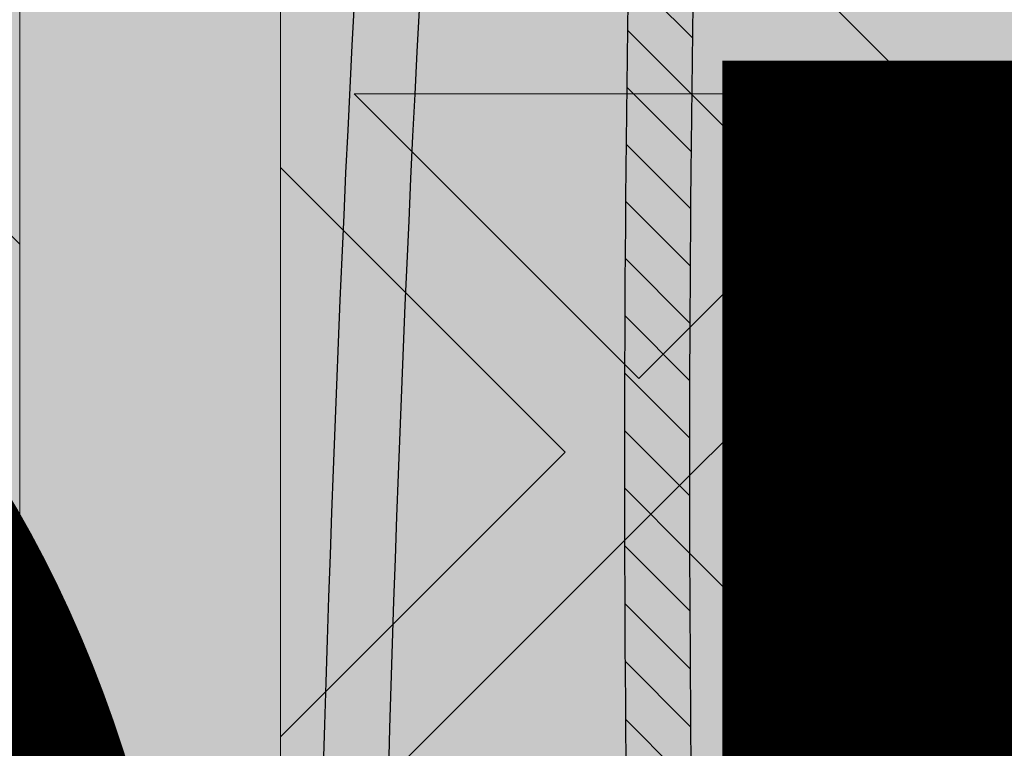
# Model space of a CAD drawing. Units: inches. Extents: x 844 to 2234, y 346 to 1084.
# Tile 77 of 93: x 1998.757 to 2001.166, y 702.727 to 704.51. Entities that reach past the tile are written whole.
import ezdxf

# ---------------------------------------------------------------- set-up
doc = ezdxf.new("R2010")
doc.units = ezdxf.units.IN
doc.header["$MEASUREMENT"] = 0
for name, color, linetype, lineweight in [('A-ANNO-DIMS', 2, 'Continuous', 18), ('furniture', 8, 'Continuous', 18), ('RA-AP-01$0$INT', 35, 'Continuous', 5)]:
    doc.layers.add(name, color=color, linetype=linetype, lineweight=lineweight)
doc.layers.add('RA-AP-01$0$FURN', color=3, linetype='Continuous')
doc.layers.add('RA-AP-01$0$WOOD', color=64, linetype='Continuous')
doc.styles.get("Standard").update_dxf_attribs({"font": 'arial.ttf'})
doc.dimstyles.get("Standard").update_dxf_attribs({"dimtxt": 6, "dimasz": 3, "dimexe": 0.18, "dimexo": 0.0625, "dimgap": 0.09, "dimtad": 0, "dimtih": 1, "dimtoh": 1, "dimdec": 1, "dimzin": 0, "dimdsep": 46, "dimlunit": 3, "dimtxsty": 'Standard', "dimblk": 'ARCHTICK', "dimcen": 0.09, "dimadec": 0, "dimazin": 0, "dimtfac": 1, "dimtdec": 1, "dimtofl": 0, "dimtmove": 0, "dimatfit": 3, "dimfxl": 1, "dimtolj": 1, "dimtzin": 0, "dimarcsym": 0})

# ---------------------------------------------------------------- blocks, each defined once
blk = doc.blocks.new('A$C18D01794')
at = {"layer": 'RA-AP-01$0$INT'}
h = blk.add_hatch(color=256, dxfattribs=at)
h.paths.add_polyline_path([(4.50521, -7.5855), (4.46935, -7.54964), (4.50521, -7.51378), (4.50521, -7.38196), (4.46935, -7.34611), (4.50521, -7.31025), (4.50521, -7.17843), (4.46935, -7.14257), (4.50521, -7.10671), (4.47692, -7.10671), (4.45521, -7.12843), (4.43349, -7.10671), (4.40521, -7.10671), (4.44106, -7.14257), (4.40521, -7.17843), (4.40521, -7.31025), (4.44106, -7.34611), (4.40521, -7.38196), (4.40521, -7.51378), (4.44106, -7.54964), (4.40521, -7.5855), (4.40521, -7.71732), (4.44106, -7.75318), (4.40521, -7.78903), (4.40521, -8.00671), (4.64435, -8.00671), (4.68021, -7.97085), (4.71606, -8.00671), (4.86935, -8.00671), (4.90521, -7.97085), (4.94106, -8.00671), (5.09435, -8.00671), (5.13021, -7.97085), (5.16606, -8.00671), (5.40521, -8.00671), (5.40521, -7.78903), (5.36935, -7.75318), (5.40521, -7.71732), (5.40521, -7.5855), (5.36935, -7.54964), (5.40521, -7.51378), (5.40521, -7.38196), (5.36935, -7.34611), (5.40521, -7.31025), (5.40521, -7.17843), (5.36935, -7.14257), (5.40521, -7.10671), (5.37692, -7.10671), (5.35521, -7.12843), (5.33349, -7.10671), (5.30521, -7.10671), (5.34106, -7.14257), (5.30521, -7.17843), (5.30521, -7.31025), (5.34106, -7.34611), (5.30521, -7.38196), (5.30521, -7.51378), (5.34106, -7.54964), (5.30521, -7.5855), (5.30521, -7.71732), (5.34106, -7.75318), (5.30521, -7.78903), (5.30521, -7.90671), (5.16606, -7.90671), (5.13021, -7.94257), (5.09435, -7.90671), (4.94106, -7.90671), (4.90521, -7.94257), (4.86935, -7.90671), (4.71606, -7.90671), (4.68021, -7.94257), (4.64435, -7.90671), (4.50521, -7.90671), (4.50521, -7.78903), (4.46935, -7.75318), (4.50521, -7.71732)])
h.paths.add_polyline_path([(4.48521, -7.70903), (4.45521, -7.73903), (4.42521, -7.70903), (4.42521, -7.59378), (4.45521, -7.56378), (4.48521, -7.59378)], flags=16)
h.paths.add_polyline_path([(4.45521, -7.76732), (4.48521, -7.79732), (4.48521, -7.91257), (4.45521, -7.94257), (4.42521, -7.91257), (4.42521, -7.79732)], flags=16)
h.paths.add_polyline_path([(4.45521, -7.5355), (4.42521, -7.5055), (4.42521, -7.39025), (4.45521, -7.36025), (4.48521, -7.39025), (4.48521, -7.5055)], flags=16)
h.paths.add_polyline_path([(4.49935, -7.92671), (4.63606, -7.92671), (4.66606, -7.95671), (4.63606, -7.98671), (4.49935, -7.98671), (4.46935, -7.95671)], flags=16)
h.paths.add_polyline_path([(4.42521, -7.94085), (4.47106, -7.98671), (4.42521, -7.98671)], flags=16)
h.paths.add_polyline_path([(4.45521, -7.33196), (4.42521, -7.30196), (4.42521, -7.18671), (4.45521, -7.15671), (4.48521, -7.18671), (4.48521, -7.30196)], flags=16)
h.paths.add_polyline_path([(4.72435, -7.92671), (4.86106, -7.92671), (4.89106, -7.95671), (4.86106, -7.98671), (4.72435, -7.98671), (4.69435, -7.95671)], flags=16)
h.paths.add_polyline_path([(4.91935, -7.95671), (4.94935, -7.92671), (5.08606, -7.92671), (5.11606, -7.95671), (5.08606, -7.98671), (4.94935, -7.98671)], flags=16)
h.paths.add_polyline_path([(5.14435, -7.95671), (5.17435, -7.92671), (5.31106, -7.92671), (5.34106, -7.95671), (5.31106, -7.98671), (5.17435, -7.98671)], flags=16)
h.paths.add_polyline_path([(5.32521, -7.59378), (5.35521, -7.56378), (5.38521, -7.59378), (5.38521, -7.70903), (5.35521, -7.73903), (5.32521, -7.70903)], flags=16)
h.paths.add_polyline_path([(5.32521, -7.79732), (5.35521, -7.76732), (5.38521, -7.79732), (5.38521, -7.91257), (5.35521, -7.94257), (5.32521, -7.91257)], flags=16)
h.paths.add_polyline_path([(5.32521, -7.5055), (5.32521, -7.39025), (5.35521, -7.36025), (5.38521, -7.39025), (5.38521, -7.5055), (5.35521, -7.5355)], flags=16)
h.paths.add_polyline_path([(5.32521, -7.30196), (5.32521, -7.18671), (5.35521, -7.15671), (5.38521, -7.18671), (5.38521, -7.30196), (5.35521, -7.33196)], flags=16)
h.paths.add_polyline_path([(5.33935, -7.98671), (5.38521, -7.94085), (5.38521, -7.98671)], flags=16)
h = blk.add_hatch(color=256, dxfattribs=at)
h.paths.add_polyline_path([(4.46935, -7.14257), (4.50521, -7.17843), (4.50521, -7.10671)])
h.paths.add_polyline_path([(4.45521, -7.12843), (4.47692, -7.10671), (4.43349, -7.10671)])
h.paths.add_polyline_path([(4.40521, -7.17843), (4.44106, -7.14257), (4.40521, -7.10671)])
h.paths.add_polyline_path([(4.42521, -7.30196), (4.45521, -7.33196), (4.48521, -7.30196), (4.48521, -7.18671), (4.45521, -7.15671), (4.42521, -7.18671)])
h.paths.add_polyline_path([(4.50521, -7.38196), (4.50521, -7.31025), (4.46935, -7.34611)])
h.paths.add_polyline_path([(4.42521, -7.5055), (4.45521, -7.5355), (4.48521, -7.5055), (4.48521, -7.39025), (4.45521, -7.36025), (4.42521, -7.39025)])
h.paths.add_polyline_path([(4.42521, -7.70903), (4.45521, -7.73903), (4.48521, -7.70903), (4.48521, -7.59378), (4.45521, -7.56378), (4.42521, -7.59378)])
h.paths.add_polyline_path([(4.46935, -7.54964), (4.50521, -7.5855), (4.50521, -7.51378)])
h.paths.add_polyline_path([(4.40521, -7.5855), (4.44106, -7.54964), (4.40521, -7.51378)])
h.paths.add_polyline_path([(4.40521, -7.78903), (4.44106, -7.75318), (4.40521, -7.71732)])
h.paths.add_polyline_path([(4.46935, -7.75318), (4.50521, -7.78903), (4.50521, -7.71732)])
h.paths.add_polyline_path([(4.42521, -7.91257), (4.45521, -7.94257), (4.48521, -7.91257), (4.48521, -7.79732), (4.45521, -7.76732), (4.42521, -7.79732)])
h.paths.add_polyline_path([(4.42521, -7.98671), (4.47106, -7.98671), (4.42521, -7.94085)])
h.paths.add_polyline_path([(4.49935, -7.98671), (4.63606, -7.98671), (4.66606, -7.95671), (4.63606, -7.92671), (4.49935, -7.92671), (4.46935, -7.95671)])
h.paths.add_polyline_path([(4.68021, -7.94257), (4.71606, -7.90671), (4.64435, -7.90671)])
h.paths.add_polyline_path([(4.64435, -8.00671), (4.71606, -8.00671), (4.68021, -7.97085)])
h.paths.add_polyline_path([(4.72435, -7.98671), (4.86106, -7.98671), (4.89106, -7.95671), (4.86106, -7.92671), (4.72435, -7.92671), (4.69435, -7.95671)])
h.paths.add_polyline_path([(4.90521, -7.94257), (4.94106, -7.90671), (4.86935, -7.90671)])
h.paths.add_polyline_path([(4.86935, -8.00671), (4.94106, -8.00671), (4.90521, -7.97085)])
h.paths.add_polyline_path([(4.94935, -7.98671), (5.08606, -7.98671), (5.11606, -7.95671), (5.08606, -7.92671), (4.94935, -7.92671), (4.91935, -7.95671)])
h.paths.add_polyline_path([(5.13021, -7.94257), (5.16606, -7.90671), (5.09435, -7.90671)])
h.paths.add_polyline_path([(5.09435, -8.00671), (5.16606, -8.00671), (5.13021, -7.97085)])
h.paths.add_polyline_path([(5.17435, -7.98671), (5.31106, -7.98671), (5.34106, -7.95671), (5.31106, -7.92671), (5.17435, -7.92671), (5.14435, -7.95671)])
h.paths.add_polyline_path([(5.32521, -7.91257), (5.35521, -7.94257), (5.38521, -7.91257), (5.38521, -7.79732), (5.35521, -7.76732), (5.32521, -7.79732)])
h.paths.add_polyline_path([(5.33935, -7.98671), (5.38521, -7.98671), (5.38521, -7.94085)])
h.paths.add_polyline_path([(5.32521, -7.70903), (5.35521, -7.73903), (5.38521, -7.70903), (5.38521, -7.59378), (5.35521, -7.56378), (5.32521, -7.59378)])
h.paths.add_polyline_path([(5.30521, -7.78903), (5.34106, -7.75318), (5.30521, -7.71732)])
h.paths.add_polyline_path([(5.36935, -7.75318), (5.40521, -7.78903), (5.40521, -7.71732)])
h.paths.add_polyline_path([(5.40521, -7.5855), (5.40521, -7.51378), (5.36935, -7.54964)])
h.paths.add_polyline_path([(5.30521, -7.5855), (5.34106, -7.54964), (5.30521, -7.51378)])
h.paths.add_polyline_path([(5.32521, -7.5055), (5.35521, -7.5355), (5.38521, -7.5055), (5.38521, -7.39025), (5.35521, -7.36025), (5.32521, -7.39025)])
h.paths.add_polyline_path([(5.30521, -7.38196), (5.34106, -7.34611), (5.30521, -7.31025)])
h.paths.add_polyline_path([(5.32521, -7.30196), (5.35521, -7.33196), (5.38521, -7.30196), (5.38521, -7.18671), (5.35521, -7.15671), (5.32521, -7.18671)])
h.paths.add_polyline_path([(5.40458, -7.38134, -0.001218), (5.40521, -7.38111), (5.40521, -7.31025), (5.36935, -7.34611)])
h.paths.add_polyline_path([(5.36935, -7.14257), (5.40521, -7.17843), (5.40521, -7.10671)])
h.paths.add_polyline_path([(5.35521, -7.12843), (5.37692, -7.10671), (5.33349, -7.10671)])
h.paths.add_polyline_path([(5.30521, -7.17843), (5.34106, -7.14257), (5.30521, -7.10671)])
blk.add_hatch(color=256, dxfattribs=at).paths.add_polyline_path([(4.50521, -7.90671), (5.30521, -7.90671), (5.30521, -7.10671), (5.25521, -7.10671), (5.25521, -7.85671), (4.55521, -7.85671), (4.55521, -7.10671), (4.50521, -7.10671)])
h = blk.add_hatch(color=256, dxfattribs=at)
h.paths.add_polyline_path([(4.58592, -7.85671), (4.6142, -7.85671), (4.66885, -7.80207), (4.72349, -7.85671), (4.77177, -7.85671), (4.82642, -7.80207), (4.86278, -7.83843), (4.8445, -7.85671), (4.86278, -7.85671), (4.90521, -7.81429), (4.94763, -7.85671), (4.96592, -7.85671), (4.94763, -7.83843), (4.98399, -7.80207), (5.03864, -7.85671), (5.08692, -7.85671), (5.14157, -7.80207), (5.19621, -7.85671), (5.2245, -7.85671), (4.90521, -7.53742)])
h.paths.add_polyline_path([(4.89521, -7.57571), (4.89521, -7.685), (4.84056, -7.63035)], flags=16)
h.paths.add_polyline_path([(4.91521, -7.57571), (4.96985, -7.63035), (4.91521, -7.685)], flags=16)
h.paths.add_polyline_path([(4.82642, -7.64449), (4.88106, -7.69914), (4.77177, -7.69914)], flags=16)
h.paths.add_polyline_path([(4.98399, -7.64449), (5.03864, -7.69914), (4.92935, -7.69914)], flags=16)
h.paths.add_polyline_path([(4.88106, -7.71914), (4.82642, -7.77378), (4.77177, -7.71914)], flags=16)
h.paths.add_polyline_path([(4.92935, -7.71914), (5.03864, -7.71914), (4.98399, -7.77378)], flags=16)
h.paths.add_polyline_path([(4.89521, -7.73328), (4.89521, -7.806), (4.87692, -7.82429), (4.84056, -7.78793)], flags=16)
h.paths.add_polyline_path([(4.91521, -7.73328), (4.96985, -7.78793), (4.93349, -7.82429), (4.91521, -7.806)], flags=16)
h.paths.add_polyline_path([(4.75763, -7.73328), (4.81228, -7.78793), (4.75763, -7.84257)], flags=16)
h.paths.add_polyline_path([(4.73763, -7.73328), (4.73763, -7.84257), (4.68299, -7.78793)], flags=16)
h.paths.add_polyline_path([(5.05278, -7.73328), (5.05278, -7.84257), (4.99814, -7.78793)], flags=16)
h.paths.add_polyline_path([(5.07278, -7.73328), (5.12742, -7.78793), (5.07278, -7.84257)], flags=16)
h.paths.add_polyline_path([(4.93592, -7.50671), (5.25521, -7.826), (5.25521, -7.79772), (5.20056, -7.74307), (5.25521, -7.68843), (5.25521, -7.64014), (5.20056, -7.5855), (5.23692, -7.54914), (5.25521, -7.56742), (5.25521, -7.54914), (5.21278, -7.50671), (5.25521, -7.46429), (5.25521, -7.446), (5.23692, -7.46429), (5.20056, -7.42793), (5.25521, -7.37328), (5.25521, -7.325), (5.20056, -7.27035), (5.25521, -7.21571), (5.25521, -7.18742)])
h.paths.add_polyline_path([(5.04299, -7.42793), (5.09763, -7.37328), (5.09763, -7.48257)], flags=16)
h.paths.add_polyline_path([(5.02885, -7.44207), (5.08349, -7.49671), (4.9742, -7.49671)], flags=16)
h.paths.add_polyline_path([(5.11763, -7.37328), (5.17228, -7.42793), (5.11763, -7.48257)], flags=16)
h.paths.add_polyline_path([(5.08349, -7.51671), (5.02885, -7.57136), (4.9742, -7.51671)], flags=16)
h.paths.add_polyline_path([(5.13177, -7.35914), (5.18642, -7.41378), (5.24106, -7.35914)], flags=17)
h.paths.add_polyline_path([(5.13177, -7.49671), (5.18642, -7.44207), (5.22278, -7.47843), (5.2045, -7.49671)], flags=16)
h.paths.add_polyline_path([(5.09763, -7.53085), (5.09763, -7.64014), (5.04299, -7.5855)], flags=16)
h.paths.add_polyline_path([(5.13177, -7.33914), (5.24106, -7.33914), (5.18642, -7.28449)], flags=17)
h.paths.add_polyline_path([(5.13177, -7.51671), (5.2045, -7.51671), (5.22278, -7.535), (5.18642, -7.57136)], flags=16)
h.paths.add_polyline_path([(5.11763, -7.53085), (5.17228, -7.5855), (5.11763, -7.64014)], flags=16)
h.paths.add_polyline_path([(5.18642, -7.59964), (5.24106, -7.65429), (5.13177, -7.65429)], flags=16)
h.paths.add_polyline_path([(5.13177, -7.67429), (5.24106, -7.67429), (5.18642, -7.72893)], flags=16)
h.paths.add_polyline_path([(5.25521, -7.126), (5.25521, -7.10671), (4.55521, -7.10671), (4.55521, -7.126), (4.90521, -7.476)])
h.paths.add_polyline_path([(4.98399, -7.36893), (4.92935, -7.31429), (5.03864, -7.31429)], flags=16)
h.paths.add_polyline_path([(4.96985, -7.38307), (4.91521, -7.43772), (4.91521, -7.32843)], flags=16)
h.paths.add_polyline_path([(4.92935, -7.29429), (4.98399, -7.23964), (5.03864, -7.29429)], flags=16)
h.paths.add_polyline_path([(5.05278, -7.28014), (4.99814, -7.2255), (5.05278, -7.17085)], flags=16)
h.paths.add_polyline_path([(5.07278, -7.28014), (5.07278, -7.17085), (5.12742, -7.2255)], flags=16)
h.paths.add_polyline_path([(4.89521, -7.43772), (4.84056, -7.38307), (4.89521, -7.32843)], flags=16)
h.paths.add_polyline_path([(4.91521, -7.28014), (4.91521, -7.20742), (4.93349, -7.18914), (4.96985, -7.2255)], flags=16)
h.paths.add_polyline_path([(4.88106, -7.31429), (4.82642, -7.36893), (4.77177, -7.31429)], flags=16)
h.paths.add_polyline_path([(4.89521, -7.28014), (4.84056, -7.2255), (4.87692, -7.18914), (4.89521, -7.20742)], flags=16)
h.paths.add_polyline_path([(4.98399, -7.21136), (4.94763, -7.175), (4.96592, -7.15671), (5.03864, -7.15671)], flags=16)
h.paths.add_polyline_path([(4.88106, -7.29429), (4.77177, -7.29429), (4.82642, -7.23964)], flags=16)
h.paths.add_polyline_path([(4.90521, -7.19914), (4.86278, -7.15671), (4.94763, -7.15671)], flags=16)
h.paths.add_polyline_path([(5.14157, -7.21136), (5.08692, -7.15671), (5.19621, -7.15671)], flags=16)
h.paths.add_polyline_path([(4.82642, -7.21136), (4.77177, -7.15671), (4.8445, -7.15671), (4.86278, -7.175)], flags=16)
h.paths.add_polyline_path([(4.81228, -7.2255), (4.75763, -7.28014), (4.75763, -7.17085)], flags=16)
h.paths.add_polyline_path([(4.73763, -7.28014), (4.68299, -7.2255), (4.73763, -7.17085)], flags=16)
h.paths.add_polyline_path([(4.72349, -7.15671), (4.66885, -7.21136), (4.6142, -7.15671)], flags=16)
h.paths.add_polyline_path([(4.59763, -7.50671), (4.55521, -7.54914), (4.55521, -7.56742), (4.57349, -7.54914), (4.60985, -7.5855), (4.55521, -7.64014), (4.55521, -7.68843), (4.60985, -7.74307), (4.55521, -7.79772), (4.55521, -7.826), (4.8745, -7.50671), (4.55521, -7.18742), (4.55521, -7.21571), (4.60985, -7.27035), (4.55521, -7.325), (4.55521, -7.37328), (4.60985, -7.42793), (4.57349, -7.46429), (4.55521, -7.446), (4.55521, -7.46429)])
h.paths.add_polyline_path([(4.71278, -7.48257), (4.71278, -7.37328), (4.76742, -7.42793)], flags=16)
h.paths.add_polyline_path([(4.72692, -7.49671), (4.78157, -7.44207), (4.83621, -7.49671)], flags=16)
h.paths.add_polyline_path([(4.69278, -7.48257), (4.63814, -7.42793), (4.69278, -7.37328)], flags=16)
h.paths.add_polyline_path([(4.72692, -7.51671), (4.83621, -7.51671), (4.78157, -7.57136)], flags=16)
h.paths.add_polyline_path([(4.67864, -7.49671), (4.60592, -7.49671), (4.58763, -7.47843), (4.62399, -7.44207)], flags=16)
h.paths.add_polyline_path([(4.71278, -7.53085), (4.76742, -7.5855), (4.71278, -7.64014)], flags=16)
h.paths.add_polyline_path([(4.67864, -7.51671), (4.62399, -7.57136), (4.58763, -7.535), (4.60592, -7.51671)], flags=16)
h.paths.add_polyline_path([(4.69278, -7.53085), (4.69278, -7.64014), (4.63814, -7.5855)], flags=16)
h.paths.add_polyline_path([(4.62399, -7.41378), (4.67864, -7.35914), (4.56935, -7.35914)], flags=17)
h.paths.add_polyline_path([(4.62399, -7.59964), (4.67864, -7.65429), (4.56935, -7.65429)], flags=16)
h.paths.add_polyline_path([(4.67864, -7.33914), (4.62399, -7.28449), (4.56935, -7.33914)], flags=17)
h.paths.add_polyline_path([(4.67864, -7.67429), (4.62399, -7.72893), (4.56935, -7.67429)], flags=16)
h = blk.add_hatch(color=256, dxfattribs=at)
h.paths.add_polyline_path([(4.90521, -7.53742), (4.8745, -7.50671), (4.55521, -7.826), (4.55521, -7.85671), (4.58592, -7.85671)])
h.paths.add_polyline_path([(4.93592, -7.50671), (4.90521, -7.53742), (5.2245, -7.85671), (5.25521, -7.85671), (5.25521, -7.826)])
h.paths.add_polyline_path([(5.25521, -7.18742), (5.25521, -7.126), (4.90521, -7.476), (4.93592, -7.50671)])
h.paths.add_polyline_path([(4.8745, -7.50671), (4.90521, -7.476), (4.55521, -7.126), (4.55521, -7.18742)])
h = blk.add_hatch(color=256, dxfattribs=at)
h.paths.add_polyline_path([(4.89521, -7.32843), (4.84056, -7.38307), (4.89521, -7.43772)])
h.paths.add_polyline_path([(4.91521, -7.43772), (4.96985, -7.38307), (4.91521, -7.32843)])
h.paths.add_polyline_path([(4.92935, -7.31429), (4.98399, -7.36893), (5.03864, -7.31429)])
h.paths.add_polyline_path([(5.03864, -7.29429), (4.98399, -7.23964), (4.92935, -7.29429)])
h.paths.add_polyline_path([(4.96985, -7.2255), (4.93349, -7.18914), (4.91521, -7.20742), (4.91521, -7.28014)])
h.paths.add_polyline_path([(4.96592, -7.15671), (4.94763, -7.175), (4.98399, -7.21136), (5.03864, -7.15671)])
h.paths.add_polyline_path([(4.99814, -7.2255), (5.05278, -7.28014), (5.05278, -7.17085)])
h.paths.add_polyline_path([(5.07278, -7.28014), (5.12742, -7.2255), (5.07278, -7.17085)])
h.paths.add_polyline_path([(5.19621, -7.15671), (5.08692, -7.15671), (5.14157, -7.21136)])
h.paths.add_polyline_path([(4.86278, -7.15671), (4.90521, -7.19914), (4.94763, -7.15671)])
h.paths.add_polyline_path([(4.89521, -7.28014), (4.89521, -7.20742), (4.87692, -7.18914), (4.84056, -7.2255)])
h.paths.add_polyline_path([(4.82642, -7.23964), (4.77177, -7.29429), (4.88106, -7.29429)])
h.paths.add_polyline_path([(4.77177, -7.31429), (4.82642, -7.36893), (4.88106, -7.31429)])
h.paths.add_polyline_path([(4.75763, -7.28014), (4.81228, -7.2255), (4.75763, -7.17085)])
h.paths.add_polyline_path([(4.86278, -7.175), (4.8445, -7.15671), (4.77177, -7.15671), (4.82642, -7.21136)])
h.paths.add_polyline_path([(4.68299, -7.2255), (4.73763, -7.28014), (4.73763, -7.17085)])
h.paths.add_polyline_path([(4.72349, -7.15671), (4.6142, -7.15671), (4.66885, -7.21136)])
h = blk.add_hatch(color=256, dxfattribs=at)
h.paths.add_polyline_path([(5.02885, -7.57136), (4.9742, -7.51671), (5.08349, -7.51671)])
h.paths.add_polyline_path([(4.9742, -7.49671), (5.02885, -7.44207), (5.08349, -7.49671)])
h.paths.add_polyline_path([(5.04299, -7.42793), (5.09763, -7.37328), (5.09763, -7.48257)])
h.paths.add_polyline_path([(5.11763, -7.48257), (5.11763, -7.37328), (5.17228, -7.42793)])
h.paths.add_polyline_path([(5.13177, -7.49671), (5.18642, -7.44207), (5.22278, -7.47843), (5.2045, -7.49671)])
h.paths.add_polyline_path([(5.23692, -7.46429), (5.20056, -7.42793), (5.25521, -7.37328), (5.25521, -7.446)])
h.paths.add_polyline_path([(5.18642, -7.41378), (5.13177, -7.35914), (5.24106, -7.35914)])
h.paths.add_polyline_path([(5.13177, -7.33914), (5.18642, -7.28449), (5.24106, -7.33914)])
h.paths.add_polyline_path([(5.20056, -7.27035), (5.25521, -7.21571), (5.25521, -7.325)])
h.paths.add_polyline_path([(5.21278, -7.50671), (5.25521, -7.46429), (5.25521, -7.54914)])
h.paths.add_polyline_path([(5.13177, -7.51671), (5.2045, -7.51671), (5.22278, -7.535), (5.18642, -7.57136)])
h.paths.add_polyline_path([(5.11763, -7.64014), (5.11763, -7.53085), (5.17228, -7.5855)])
h.paths.add_polyline_path([(5.04299, -7.5855), (5.09763, -7.53085), (5.09763, -7.64014)])
h.paths.add_polyline_path([(5.13177, -7.65429), (5.18642, -7.59964), (5.24106, -7.65429)])
h.paths.add_polyline_path([(5.20056, -7.5855), (5.23692, -7.54914), (5.25521, -7.56742), (5.25521, -7.64014)])
h.paths.add_polyline_path([(5.18642, -7.72893), (5.13177, -7.67429), (5.24106, -7.67429)])
h.paths.add_polyline_path([(5.20056, -7.74307), (5.25521, -7.68843), (5.25521, -7.79772)])
for p, q in [((5.25521, -7.10671), (5.25521, -7.85671)), ((4.90521, -7.476), (5.25521, -7.126)), ((5.07278, -7.17085), (5.12742, -7.2255)), ((4.93592, -7.50671), (5.25521, -7.18742)), ((5.25521, -7.21571), (5.20056, -7.27035)), ((5.25521, -7.325), (5.25521, -7.21571)), ((5.12742, -7.2255), (5.07278, -7.28014)), ((5.25521, -7.325), (5.20056, -7.27035)), ((5.18642, -7.28449), (5.13177, -7.33914)), ((5.24106, -7.33914), (5.18642, -7.28449)), ((5.30521, -7.31025), (5.34106, -7.34611)), ((5.13177, -7.33914), (5.24106, -7.33914))]:
    blk.add_line(p, q, dxfattribs=at)
blk.add_lwpolyline([(5.30521, -7.10671), (5.30521, -7.90671), (4.50521, -7.90671), (4.50521, -7.10671)], dxfattribs=at)
blk = doc.blocks.new('A$C32926AE1')
at = {"layer": 'RA-AP-01$0$WOOD'}
h = blk.add_hatch(color=256, dxfattribs=at)
h.dxf.hatch_style = 1
h.paths.add_polyline_path([(5.15743, 4.57348, -0.100949), (5.1554, 4.59337, -0.184266), (5.17225, 4.6388, 0.205661), (5.17956, 4.66132, 0.361434), (5.13435, 4.70652, 0.205661), (5.11183, 4.69921, -0.184266), (5.0664, 4.68237, -0.105531), (5.04566, 4.68467, 0.156764), (4.76389, 4.68467, -0.105531), (4.74314, 4.68237, -0.184266), (4.69771, 4.69921, 0.205661), (4.67519, 4.70652, 0.361434), (4.62998, 4.66132, 0.205661), (4.63729, 4.6388, -0.184266), (4.65414, 4.59337, -0.100949), (4.65211, 4.57348, 0.02141), (4.62975, 4.15671, 0.02141), (4.65211, 3.73994, -0.100949), (4.65414, 3.72006, -0.184266), (4.63729, 3.67463, 0.205661), (4.62998, 3.65211, 0.361434), (4.67519, 3.6069, 0.205661), (4.69771, 3.61421, -0.184266), (4.74314, 3.63106, -0.105531), (4.76389, 3.62875, 0.156764), (5.04566, 3.62875, -0.105531), (5.0664, 3.63106, -0.184266), (5.11183, 3.61421, 0.205661), (5.13435, 3.6069, 0.361434), (5.17956, 3.65211, 0.205661), (5.17225, 3.67463, -0.184266), (5.1554, 3.72006, -0.100949), (5.15743, 3.73994, 0.02141), (5.17979, 4.15671, 0.02141)])
h.paths.add_polyline_path([(4.63975, 4.15671, 0.021354), (4.66197, 3.74189, -0.094076), (4.66414, 3.71961, -0.182482), (4.64481, 3.66804, 0.205661), (4.63994, 3.65302, 0.361434), (4.67611, 3.61686, 0.205661), (4.69112, 3.62173, -0.182482), (4.7427, 3.64106, -0.102989), (4.76699, 3.63826, 0.156709), (5.04255, 3.63826, -0.102989), (5.06685, 3.64106, -0.182482), (5.11842, 3.62173, 0.205661), (5.13344, 3.61686, 0.361434), (5.1696, 3.65302, 0.205661), (5.16473, 3.66804, -0.182482), (5.1454, 3.71961, -0.094076), (5.14757, 3.74189, 0.021354), (5.16979, 4.15671, 0.021354), (5.14757, 4.57154, -0.094076), (5.1454, 4.59381, -0.182482), (5.16473, 4.64539, 0.205661), (5.1696, 4.6604, 0.361434), (5.13344, 4.69657, 0.205661), (5.11842, 4.69169, -0.182482), (5.06685, 4.67236, -0.102989), (5.04255, 4.67517, 0.156709), (4.76699, 4.67517, -0.102989), (4.7427, 4.67236, -0.182482), (4.69112, 4.69169, 0.205661), (4.67611, 4.69657, 0.361434), (4.63994, 4.6604, 0.205661), (4.64481, 4.64539, -0.182482), (4.66414, 4.59381, -0.094076), (4.66197, 4.57154, 0.021354)], flags=16)
h.paths.add_polyline_path([(5.12979, 4.43217, -0.014166), (5.13015, 4.15693, -0.014166), (5.12979, 3.88169, -0.078525), (5.1098, 3.75514, 0.094597), (5.10541, 3.7179, 0.104317), (5.11607, 3.67039, 0.104317), (5.06856, 3.68105, 0.094597), (5.03132, 3.67666, -0.158024), (4.77823, 3.67666, 0.094597), (4.74098, 3.68105, 0.104317), (4.69347, 3.67039, 0.104317), (4.70413, 3.7179, 0.094597), (4.69975, 3.75514, -0.078525), (4.67975, 3.88169, -0.014166), (4.67939, 4.15693, -0.014166), (4.67975, 4.43217, -0.078525), (4.69975, 4.55871, 0.094597), (4.70413, 4.59596, 0.104317), (4.69347, 4.64347, 0.104317), (4.74098, 4.6328, 0.094597), (4.77823, 4.63719, -0.158024), (5.03132, 4.63719, 0.094597), (5.06856, 4.6328, 0.104317), (5.11607, 4.64347, 0.104317), (5.10541, 4.59596, 0.094597), (5.1098, 4.55871, -0.078525)], flags=0)
h.paths.add_polyline_path([(5.11979, 4.43226, -0.0142), (5.12016, 4.15693, -0.0142), (5.11979, 3.8816, -0.078489), (5.10027, 3.75819, 0.094014), (5.09541, 3.71748, 0.060627), (5.09962, 3.68684, 0.060627), (5.06898, 3.69105, 0.094014), (5.02827, 3.68619, -0.158071), (4.78127, 3.68619, 0.094014), (4.74056, 3.69105, 0.060627), (4.70993, 3.68684, 0.060627), (4.71413, 3.71748, 0.094014), (4.70927, 3.75819, -0.078489), (4.68975, 3.8816, -0.0142), (4.68939, 4.15693, -0.0142), (4.68975, 4.43226, -0.078489), (4.70927, 4.55566, 0.094014), (4.71413, 4.59638, 0.060627), (4.70993, 4.62701, 0.060627), (4.74056, 4.62281, 0.094014), (4.78127, 4.62767, -0.158071), (5.02827, 4.62767, 0.094014), (5.06898, 4.62281, 0.060627), (5.09962, 4.62701, 0.060627), (5.09541, 4.59638, 0.094014), (5.10027, 4.55566, -0.078489)], flags=0)
h.paths.add_polyline_path([(5.06979, 4.43022, -0.014242), (5.07017, 4.15693, -0.014242), (5.06979, 3.88364, -0.080061), (5.05266, 3.77346, 0.052642), (5.04591, 3.74055, 0.052642), (5.013, 3.7338, -0.158303), (4.79655, 3.7338, 0.052642), (4.76363, 3.74055, 0.052642), (4.75688, 3.77346, -0.080061), (4.73975, 3.88364, -0.014242), (4.73937, 4.15693, -0.014242), (4.73975, 4.43022, -0.080061), (4.75688, 4.54039, 0.052642), (4.76363, 4.5733, 0.052642), (4.79655, 4.58006, -0.158303), (5.013, 4.58006, 0.052642), (5.04591, 4.5733, 0.052642), (5.05266, 4.54039, -0.080061)], flags=0)
h.paths.add_polyline_path([(5.04979, 4.43038, -0.01431), (5.05018, 4.15693, -0.01431), (5.04979, 3.88347, -0.080069), (5.03362, 3.77958, 0.030626), (5.02824, 3.75822, 0.030626), (5.00688, 3.75284, -0.158398), (4.80266, 3.75284, 0.030626), (4.7813, 3.75822, 0.030626), (4.77592, 3.77958, -0.080069), (4.75975, 3.88347, -0.01431), (4.75936, 4.15693, -0.01431), (4.75975, 4.43038, -0.080069), (4.77592, 4.53427, 0.030626), (4.7813, 4.55564, 0.030626), (4.80266, 4.56102, -0.158398), (5.00688, 4.56102, 0.030626), (5.02824, 4.55564, 0.030626), (5.03362, 4.53427, -0.080069)], flags=0)
h.paths.add_polyline_path([(4.99977, 4.42817, -0.014344), (5.0002, 4.15693, -0.014344), (4.99977, 3.88568, -0.078464), (4.98736, 3.7991, -0.150605), (4.82219, 3.7991, -0.078464), (4.80978, 3.88568, -0.014344), (4.80934, 4.15693, -0.014344), (4.80978, 4.42817, -0.078464), (4.82219, 4.51475, -0.150605), (4.98736, 4.51475, -0.078464)], flags=0)
h.paths.add_polyline_path([(4.97976, 4.42764, -0.014377), (4.98021, 4.15693, -0.014377), (4.97976, 3.88621, -0.068924), (4.97118, 3.81528, -0.129665), (4.83836, 3.81528, -0.068924), (4.82979, 3.88621, -0.014377), (4.82934, 4.15693, -0.014377), (4.82979, 4.42764, -0.068924), (4.83836, 4.49858, -0.129665), (4.97118, 4.49858, -0.068924)], flags=0)
h = blk.add_hatch(color=256, dxfattribs=at)
h.dxf.hatch_style = 1
h.paths.add_polyline_path([(5.1454, 4.59381, -0.182482), (5.16473, 4.64539, 0.205661), (5.1696, 4.6604, 0.361434), (5.13344, 4.69657, 0.205661), (5.11842, 4.69169, -0.182482), (5.06685, 4.67236, -0.102989), (5.04255, 4.67517, 0.156709), (4.76699, 4.67517, -0.102989), (4.7427, 4.67236, -0.182482), (4.69112, 4.69169, 0.205661), (4.67611, 4.69657, 0.361434), (4.63994, 4.6604, 0.205661), (4.64481, 4.64539, -0.182482), (4.66414, 4.59381, -0.094076), (4.66197, 4.57154, 0.021354), (4.63975, 4.15671, 0.021354), (4.66197, 3.74189, -0.094076), (4.66414, 3.71961, -0.182482), (4.64481, 3.66804, 0.205661), (4.63994, 3.65302, 0.361434), (4.67611, 3.61686, 0.205661), (4.69112, 3.62173, -0.182482), (4.7427, 3.64106, -0.102989), (4.76699, 3.63826, 0.156709), (5.04255, 3.63826, -0.102989), (5.06685, 3.64106, -0.182482), (5.11842, 3.62173, 0.205661), (5.13344, 3.61686, 0.361434), (5.1696, 3.65302, 0.205661), (5.16473, 3.66804, -0.182482), (5.1454, 3.71961, -0.094076), (5.14757, 3.74189, 0.021354), (5.16979, 4.15671, 0.021354), (5.14757, 4.57154, -0.094076)])
h.paths.add_polyline_path([(5.1098, 4.55871, -0.078525), (5.12979, 4.43217, -0.014166), (5.13015, 4.15693, -0.014166), (5.12979, 3.88169, -0.078525), (5.1098, 3.75514, 0.094597), (5.10541, 3.7179, 0.104317), (5.11607, 3.67039, 0.104317), (5.06856, 3.68105, 0.094597), (5.03132, 3.67666, -0.158024), (4.77823, 3.67666, 0.094597), (4.74098, 3.68105, 0.104317), (4.69347, 3.67039, 0.104317), (4.70413, 3.7179, 0.094597), (4.69975, 3.75514, -0.078525), (4.67975, 3.88169, -0.014166), (4.67939, 4.15693, -0.014166), (4.67975, 4.43217, -0.078525), (4.69975, 4.55871, 0.094597), (4.70413, 4.59596, 0.104317), (4.69347, 4.64347, 0.104317), (4.74098, 4.6328, 0.094597), (4.77823, 4.63719, -0.158024), (5.03132, 4.63719, 0.094597), (5.06856, 4.6328, 0.104317), (5.11607, 4.64347, 0.104317), (5.10541, 4.59596, 0.094597)], flags=16)
h.paths.add_polyline_path([(5.10027, 4.55566, -0.078489), (5.11979, 4.43226, -0.0142), (5.12016, 4.15693, -0.0142), (5.11979, 3.8816, -0.078489), (5.10027, 3.75819, 0.094014), (5.09541, 3.71748, 0.060627), (5.09962, 3.68684, 0.060627), (5.06898, 3.69105, 0.094014), (5.02827, 3.68619, -0.158071), (4.78127, 3.68619, 0.094014), (4.74056, 3.69105, 0.060627), (4.70993, 3.68684, 0.060627), (4.71413, 3.71748, 0.094014), (4.70927, 3.75819, -0.078489), (4.68975, 3.8816, -0.0142), (4.68939, 4.15693, -0.0142), (4.68975, 4.43226, -0.078489), (4.70927, 4.55566, 0.094014), (4.71413, 4.59638, 0.060627), (4.70993, 4.62701, 0.060627), (4.74056, 4.62281, 0.094014), (4.78127, 4.62767, -0.158071), (5.02827, 4.62767, 0.094014), (5.06898, 4.62281, 0.060627), (5.09962, 4.62701, 0.060627), (5.09541, 4.59638, 0.094014)], flags=0)
h.paths.add_polyline_path([(5.04591, 4.5733, 0.052642), (5.05266, 4.54039, -0.080061), (5.06979, 4.43022, -0.014242), (5.07017, 4.15693, -0.014242), (5.06979, 3.88364, -0.080061), (5.05266, 3.77346, 0.052642), (5.04591, 3.74055, 0.052642), (5.013, 3.7338, -0.158303), (4.79655, 3.7338, 0.052642), (4.76363, 3.74055, 0.052642), (4.75688, 3.77346, -0.080061), (4.73975, 3.88364, -0.014242), (4.73937, 4.15693, -0.014242), (4.73975, 4.43022, -0.080061), (4.75688, 4.54039, 0.052642), (4.76363, 4.5733, 0.052642), (4.79655, 4.58006, -0.158303), (5.013, 4.58006, 0.052642)], flags=0)
h.paths.add_polyline_path([(5.02824, 4.55564, 0.030626), (5.03362, 4.53427, -0.080069), (5.04979, 4.43038, -0.01431), (5.05018, 4.15693, -0.01431), (5.04979, 3.88347, -0.080069), (5.03362, 3.77958, 0.030626), (5.02824, 3.75822, 0.030626), (5.00688, 3.75284, -0.158398), (4.80266, 3.75284, 0.030626), (4.7813, 3.75822, 0.030626), (4.77592, 3.77958, -0.080069), (4.75975, 3.88347, -0.01431), (4.75936, 4.15693, -0.01431), (4.75975, 4.43038, -0.080069), (4.77592, 4.53427, 0.030626), (4.7813, 4.55564, 0.030626), (4.80266, 4.56102, -0.158398), (5.00688, 4.56102, 0.030626)], flags=0)
h.paths.add_polyline_path([(4.98736, 4.51475, -0.078464), (4.99977, 4.42817, -0.014344), (5.0002, 4.15693, -0.014344), (4.99977, 3.88568, -0.078464), (4.98736, 3.7991, -0.150605), (4.82219, 3.7991, -0.078464), (4.80978, 3.88568, -0.014344), (4.80934, 4.15693, -0.014344), (4.80978, 4.42817, -0.078464), (4.82219, 4.51475, -0.150605)], flags=0)
h.paths.add_polyline_path([(4.97118, 4.49858, -0.068924), (4.97976, 4.42764, -0.014377), (4.98021, 4.15693, -0.014377), (4.97976, 3.88621, -0.068924), (4.97118, 3.81528, -0.129665), (4.83836, 3.81528, -0.068924), (4.82979, 3.88621, -0.014377), (4.82934, 4.15693, -0.014377), (4.82979, 4.42764, -0.068924), (4.83836, 4.49858, -0.129665)], flags=0)
h = blk.add_hatch(dxfattribs=at)
h.set_pattern_fill('ANSI31', color=256, scale=0.05, style=0)
h.paths.add_polyline_path([(5.13015, 4.15693, 0.014166), (5.12979, 4.43217, 0.077783), (5.11017, 4.55756, -0.097652), (5.10541, 4.59596, -0.104317), (5.11607, 4.64347), (5.09962, 4.62701, 0.060627), (5.09541, 4.59638, 0.094014), (5.10027, 4.55566, -0.078489), (5.11979, 4.43226, -0.0142), (5.12016, 4.15693, -0.0142), (5.11979, 3.8816, -0.078489), (5.10027, 3.75819, 0.094014), (5.09541, 3.71748, 0.060627), (5.09962, 3.68684), (5.11607, 3.67039, -0.104317), (5.10541, 3.7179, -0.097652), (5.11017, 3.7563, 0.077783), (5.12979, 3.88169, 0.014166)])
h.paths.add_polyline_path([(5.03016, 3.67629, -0.097652), (5.06856, 3.68105, -0.104317), (5.11607, 3.67039), (5.09962, 3.68684, 0.060627), (5.06898, 3.69105, 0.094014), (5.02827, 3.68619, -0.158071), (4.78127, 3.68619, 0.094014), (4.74056, 3.69105, 0.060627), (4.70993, 3.68684), (4.69347, 3.67039, -0.104317), (4.74098, 3.68105, -0.097652), (4.77938, 3.67629, 0.156513)])
h.paths.add_polyline_path([(4.68975, 3.8816, -0.0142), (4.68939, 4.15693, -0.0142), (4.68975, 4.43226, -0.078489), (4.70927, 4.55566, 0.094014), (4.71413, 4.59638, 0.060627), (4.70993, 4.62701), (4.69347, 4.64347, -0.104317), (4.70413, 4.59596, -0.097652), (4.69937, 4.55756, 0.077783), (4.67975, 4.43217, 0.014166), (4.67939, 4.15693, 0.014166), (4.67975, 3.88169, 0.077783), (4.69937, 3.7563, -0.097652), (4.70413, 3.7179, -0.104317), (4.69347, 3.67039), (4.70993, 3.68684, 0.060627), (4.71413, 3.71748, 0.094014), (4.70927, 3.75819, -0.078489)])
h.paths.add_polyline_path([(4.77938, 4.63756, -0.097652), (4.74098, 4.6328, -0.104317), (4.69347, 4.64347), (4.70993, 4.62701, 0.060627), (4.74056, 4.62281, 0.094014), (4.78127, 4.62767, -0.158071), (5.02827, 4.62767, 0.094014), (5.06898, 4.62281, 0.060627), (5.09962, 4.62701), (5.11607, 4.64347, -0.104317), (5.06856, 4.6328, -0.097652), (5.03016, 4.63756, 0.156513)])
h = blk.add_hatch(dxfattribs=at)
h.set_pattern_fill('ANSI32', color=256, scale=0.2, style=0)
h.paths.add_polyline_path([(5.11979, 4.43226, 0.077702), (5.10066, 4.55447, -0.09689), (5.09541, 4.59638, -0.060627), (5.09962, 4.62701, -0.060627), (5.06898, 4.62281, -0.09689), (5.02707, 4.62805, 0.156466), (4.78247, 4.62805, -0.09689), (4.74056, 4.62281, -0.060627), (4.70993, 4.62701, -0.060627), (4.71413, 4.59638, -0.09689), (4.70888, 4.55447, 0.077702), (4.68975, 4.43226, 0.0142), (4.68939, 4.15693, 0.0142), (4.68975, 3.8816, 0.077702), (4.70888, 3.75939, -0.09689), (4.71413, 3.71748, -0.060627), (4.70993, 3.68684, -0.060627), (4.74056, 3.69105, -0.09689), (4.78247, 3.6858, 0.156466), (5.02707, 3.6858, -0.09689), (5.06898, 3.69105, -0.060627), (5.09962, 3.68684, -0.060627), (5.09541, 3.71748, -0.09689), (5.10066, 3.75939, 0.077702), (5.11979, 3.8816, 0.0142), (5.12016, 4.15693, 0.0142)])
h.paths.add_polyline_path([(5.07017, 4.15693, -0.014242), (5.06979, 3.88364, -0.080061), (5.05266, 3.77346, 0.052642), (5.04591, 3.74055, 0.052642), (5.013, 3.7338, -0.158303), (4.79655, 3.7338, 0.052642), (4.76363, 3.74055, 0.052642), (4.75688, 3.77346, -0.080061), (4.73975, 3.88364, -0.014242), (4.73937, 4.15693, -0.014242), (4.73975, 4.43022, -0.080061), (4.75688, 4.54039, 0.052642), (4.76363, 4.5733, 0.052642), (4.79655, 4.58006, -0.158303), (5.013, 4.58006, 0.052642), (5.04591, 4.5733, 0.052642), (5.05266, 4.54039, -0.080061), (5.06979, 4.43022, -0.014242)], flags=16)
h.paths.add_polyline_path([(5.05018, 4.15693, -0.01431), (5.04979, 3.88347, -0.080069), (5.03362, 3.77958, 0.030626), (5.02824, 3.75822, 0.030626), (5.00688, 3.75284, -0.158398), (4.80266, 3.75284, 0.030626), (4.7813, 3.75822, 0.030626), (4.77592, 3.77958, -0.080069), (4.75975, 3.88347, -0.01431), (4.75936, 4.15693, -0.01431), (4.75975, 4.43038, -0.080069), (4.77592, 4.53427, 0.030626), (4.7813, 4.55564, 0.030626), (4.80266, 4.56102, -0.158398), (5.00688, 4.56102, 0.030626), (5.02824, 4.55564, 0.030626), (5.03362, 4.53427, -0.080069), (5.04979, 4.43038, -0.01431)], flags=0)
h.paths.add_polyline_path([(5.0002, 4.15693, -0.014344), (4.99977, 3.88568, -0.078464), (4.98736, 3.7991, -0.150605), (4.82219, 3.7991, -0.078464), (4.80978, 3.88568, -0.014344), (4.80934, 4.15693, -0.014344), (4.80978, 4.42817, -0.078464), (4.82219, 4.51475, -0.150605), (4.98736, 4.51475, -0.078464), (4.99977, 4.42817, -0.014344)], flags=0)
h.paths.add_polyline_path([(4.98021, 4.15693, -0.014377), (4.97976, 3.88621, -0.068924), (4.97118, 3.81528, -0.129665), (4.83836, 3.81528, -0.068924), (4.82979, 3.88621, -0.014377), (4.82934, 4.15693, -0.014377), (4.82979, 4.42764, -0.068924), (4.83836, 4.49858, -0.129665), (4.97118, 4.49858, -0.068924), (4.97976, 4.42764, -0.014377)], flags=0)
for centre, radius, start, end in [((0.30432, 4.10408), 4.87575, 0.6185, 5.52459), ((0.30432, 4.10408), 4.86575, 0.6185, 5.51296), ((0.27359, 4.28823), 4.85833, 358.45262, 1.69776), ((0.27359, 4.28823), 4.84835, 358.44816, 1.6933)]:
    blk.add_arc(centre, radius, start, end, dxfattribs=at)
blk = doc.blocks.new('A$C5D2F253E')
at = {"layer": 'RA-AP-01$0$FURN', "xscale": -0.7999999999883585, "yscale": 0.7999999999883585, "zscale": 0.8, "rotation": 90}
blk.add_blockref('A$C18D01794', (-5.68776, 4.75792), dxfattribs=at)
at = {"layer": 'RA-AP-01$0$WOOD', "rotation": 270}
blk.add_blockref('A$C32926AE1', (-4.16134, 5.73853), dxfattribs=at)
blk = doc.blocks.new('_ArchTick')
at = {"color": 0, "linetype": 'ByBlock', "const_width": 0.15}
blk.add_lwpolyline([(-0.5, -0.5), (0.5, 0.5)], dxfattribs=at)
blk = doc.blocks.new('*D121')
at = {"layer": 'A-ANNO-DIMS', "color": 0, "lineweight": -2, "transparency": 16777216}
for p, q in [((2030.272, 734.2626), (2040.2453, 734.2626)), ((2040.0653, 734.2626), (2040.0653, 704.6044)), ((2040.0653, 668.5574), (2040.0653, 698.2156)), ((2030.272, 668.5574), (2040.2453, 668.5574))]:
    blk.add_line(p, q, dxfattribs=at)
at = {"layer": 'Defpoints', "color": 0, "transparency": 16777216}
for p in [(2030.2095, 734.2626), (2040.0653, 734.2626), (2030.2095, 668.5574)]:
    blk.add_point(p, dxfattribs=at)
at = {"layer": 'A-ANNO-DIMS', "color": 0, "lineweight": -2, "transparency": 16777216, "xscale": 3, "yscale": 3, "zscale": 3}
for p, rotation in [((2040.0653, 734.2626), 90), ((2040.0653, 668.5574), 270)]:
    blk.add_blockref('_ArchTick', p, dxfattribs=dict(at, rotation=rotation))
at = {"layer": 'A-ANNO-DIMS', "color": 0, "transparency": 16777216, "insert": (2040.0653, 701.41), "char_height": 6, "attachment_point": 5}
blk.add_mtext('\\A1;LOUNGE SET 5\'-5 1/2" TYP.', dxfattribs=at)

msp = doc.modelspace()

# ---------------------------------------------------------------- block references
at = {"layer": 'furniture', "xscale": -15.94108302203742, "yscale": 15.94108302203742, "zscale": 15.94108302203742, "rotation": 270}
msp.add_blockref('A$C5D2F253E', (1990.5673, 701.4029), dxfattribs=at)

# ---------------------------------------------------------------- dimensions: what is measured, and where the dimension line sits
at = {"layer": 'A-ANNO-DIMS'}
dim = msp.add_linear_dim(base=(2040.0653, 734.2626), p1=(2030.2095, 668.5574), p2=(2030.2095, 734.2626), angle=90, text='LOUNGE SET <> TYP.', dimstyle='Standard', override={"dimdec": 1, "dimlfac": 1, "dimrnd": 0, "dimzin": 1, "dimdsep": 46, "dimlunit": 4, "dimfrac": 2}, dxfattribs=at)
dim.commit()
dim.dimension.update_dxf_attribs({"geometry": '*D121', "text_midpoint": (2040.0653, 701.41)})

doc.saveas('drawing.dxf')
